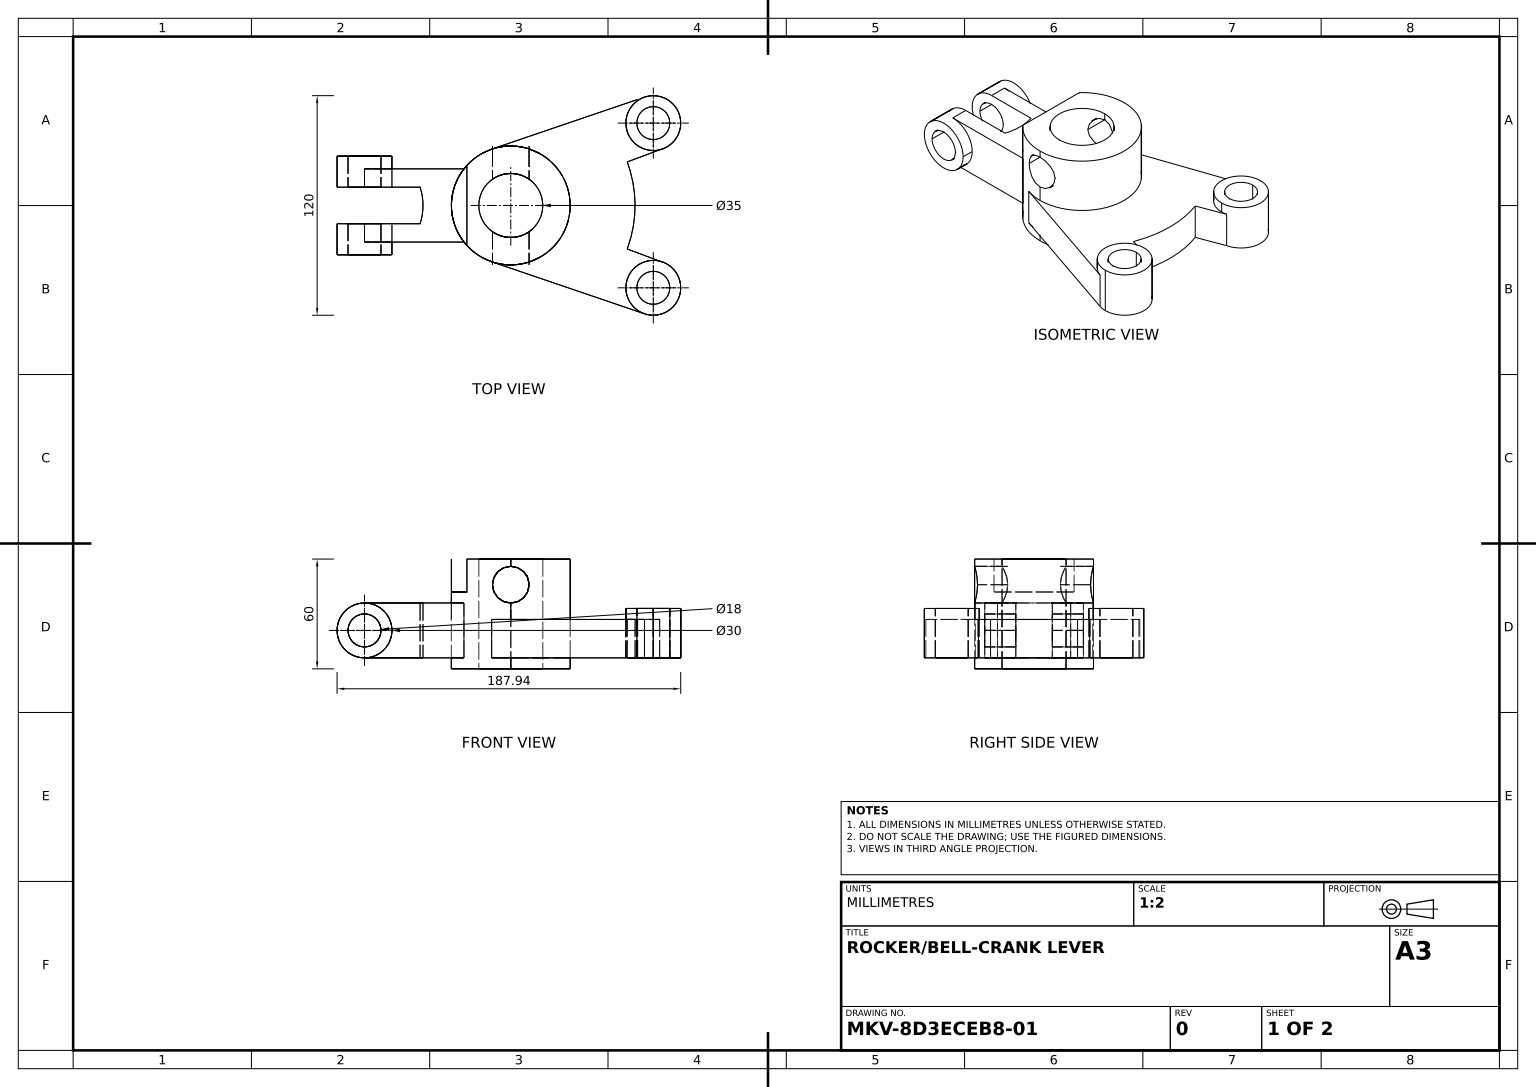
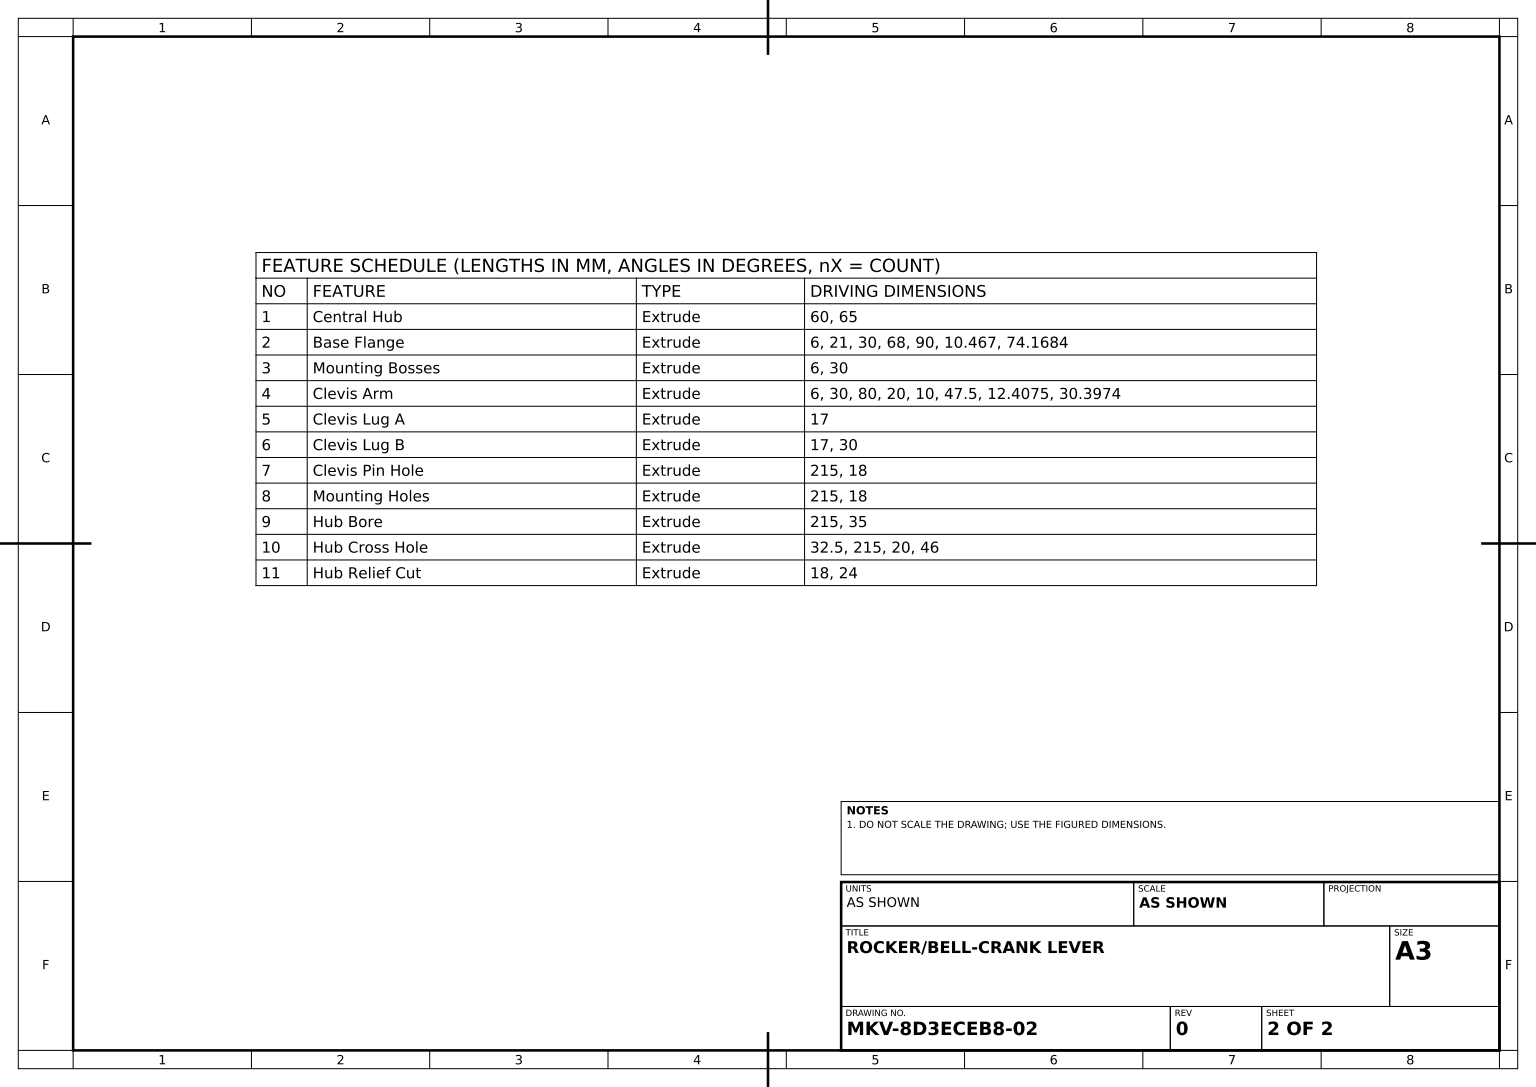
from build123d import *

# Parameters (mm, degrees)
HUB_PROFILE_SKETCH_R     = 32.5
CENTRAL_HUB_DEPTH        = 60
BASE_FLANGE_DEPTH        = 21
MOUNTING_BOSSES_SKETCH_R = 15
MOUNTING_BOSSES_DEPTH    = 6
CLEVIS_ARM_DEPTH         = 30
CLEVIS_LUG_A_SKETCH_R    = 15
CLEVIS_LUG_A_DEPTH       = 17
CLEVIS_START             = -17
CLEVIS_LUG_B_SKETCH_R    = 15
CLEVIS_LUG_B_DEPTH       = 17
CLEVIS_PIN_HOLE_SKETCH_R = 9
CLEVIS_PIN_HOLE_DEPTH    = 215
MOUNTING_HOLES_SKETCH_R  = 9
MOUNTING_HOLES_DEPTH     = 215
HUB_BORE_SKETCH_R        = 17.5
HUB_BORE_DEPTH           = 215
HUB_CROSS_HOLE_SKETCH_R  = 10
HUB_CROSS_HOLE_DEPTH     = 215
HUB_START                = -18
HUB_RELIEF_CUT_DEPTH     = 18


with BuildPart() as part:
    # Hub Profile Sketch → Central Hub (new body)
    with BuildSketch(Plane(origin=(0, 0, 0), x_dir=(1, 0, 0), z_dir=(0, 1, 0))):
        with Locations(Location((0, 0, 0), (0, 0, 270))):
            Circle(HUB_PROFILE_SKETCH_R)
    extrude(amount=CENTRAL_HUB_DEPTH)

    # Base Flange Sketch → Base Flange (add)
    with BuildSketch(Plane(origin=(0, 6, 0), x_dir=(1, 0, 0), z_dir=(0, 1, 0))):
        with BuildLine():
            Line((68.988226854, 57.798136264), (-10.467045475, 30.768343456))
            ThreePointArc((-10.467045475, 30.768343456), (32.5, 0), (-10.467045475, -30.768343456))
            Line((-10.467045475, -30.768343456), (73.111342275, -59.200773903))
            ThreePointArc((73.111342275, -59.200773903), (92.357418682, -49.147765612), (81.39742245, -30.40335537))
            Line((81.39742245, -30.40335537), (63.701379755, -23.793575127))
            ThreePointArc((63.701379755, -23.793575127), (68, 0), (63.701379755, 23.793575127))
            Line((63.701379755, 23.793575127), (81.39742245, 30.40335537))
            ThreePointArc((81.39742245, 30.40335537), (91.640276267, 51.112697602), (69.385841621, 57.320196986))
            ThreePointArc((69.385841621, 57.320196986), (69.187446933, 57.559509961), (68.988226854, 57.798136264))
        make_face()
    extrude(amount=BASE_FLANGE_DEPTH)

    # Mounting Bosses Sketch → Mounting Bosses (add)
    with BuildSketch(Plane(origin=(0, 27, 0), x_dir=(1, 0, 0), z_dir=(0, 1, 0))):
        with Locations(Location((77.942286341, 45, 0), (0, 0, 124.780191847))):
            Circle(MOUNTING_BOSSES_SKETCH_R)
        with Locations(Location((77.942286341, -45, 0), (0, 0, 76.682768473))):
            Circle(MOUNTING_BOSSES_SKETCH_R)
    extrude(amount=MOUNTING_BOSSES_DEPTH)

    # Clevis Arm Sketch → Clevis Arm (add)
    with BuildSketch(Plane(origin=(0, 6, 0), x_dir=(1, 0, 0), z_dir=(0, 1, 0))):
        with BuildLine():
            ThreePointArc((-49.602631693, -10), (-48, 0), (-49.602631693, 10))
            Line((-49.602631693, 10), (-80, 10))
            Line((-80, 10), (-80, 20))
            Line((-80, 20), (-32.5, 20))
            Line((-32.5, 20), (-20.092522132, 20))
            Line((-20.092522132, 20), (-20.092522132, -20))
            Line((-20.092522132, -20), (-32.5, -20))
            Line((-32.5, -20), (-80, -20))
            Line((-80, -20), (-80, -10))
            Line((-80, -10), (-49.602631693, -10))
        make_face()
    extrude(amount=CLEVIS_ARM_DEPTH)

    # Clevis Lug A Sketch → Clevis Lug A (add)
    with BuildSketch(Plane(origin=(0, 0, 10), x_dir=(-1, 0, 0), z_dir=(0, 0, -1))):
        with Locations((80, 21)):
            Circle(CLEVIS_LUG_A_SKETCH_R)
    extrude(amount=-CLEVIS_LUG_A_DEPTH)

    # Clevis Lug B Sketch → Clevis Lug B (add)
    with BuildSketch(Plane.XY.offset(-10).offset(CLEVIS_START)):
        with Locations(Location((-80, 21, 0), (0, 0, 180))):
            Circle(CLEVIS_LUG_B_SKETCH_R)
    extrude(amount=CLEVIS_LUG_B_DEPTH)

    # Clevis Pin Hole Sketch → Clevis Pin Hole (cut)
    with BuildSketch(Plane.XY.offset(27)):
        with Locations((-80, 21)):
            Circle(CLEVIS_PIN_HOLE_SKETCH_R)
    extrude(amount=-CLEVIS_PIN_HOLE_DEPTH, mode=Mode.SUBTRACT)

    # Mounting Holes Sketch → Mounting Holes (cut)
    with BuildSketch(Plane(origin=(0, 33, 0), x_dir=(1, 0, 0), z_dir=(0, 1, 0))):
        with Locations(Location((77.942286341, 45, 0), (0, 0, 270))):
            Circle(MOUNTING_HOLES_SKETCH_R)
        with Locations(Location((77.942286341, -45, 0), (0, 0, 270))):
            Circle(MOUNTING_HOLES_SKETCH_R)
    extrude(amount=-MOUNTING_HOLES_DEPTH, mode=Mode.SUBTRACT)

    # Hub Bore Sketch → Hub Bore (cut)
    with BuildSketch(Plane(origin=(0, 60, 0), x_dir=(1, 0, 0), z_dir=(0, 1, 0))):
        with Locations(Location((0, 0, 0), (0, 0, 270))):
            Circle(HUB_BORE_SKETCH_R)
    extrude(amount=-HUB_BORE_DEPTH, mode=Mode.SUBTRACT)

    # Hub Cross Hole Sketch → Hub Cross Hole (cut)
    with BuildSketch(Plane.XY.offset(32.5)):
        with Locations((0, 46)):
            Circle(HUB_CROSS_HOLE_SKETCH_R)
    extrude(amount=-HUB_CROSS_HOLE_DEPTH, mode=Mode.SUBTRACT)

    # Hub Relief Cut Sketch → Hub Relief Cut (cut)
    with BuildSketch(Plane(origin=(0, 60, 0), x_dir=(1, 0, 0), z_dir=(0, 1, 0)).offset(HUB_START)):
        with BuildLine():
            Line((-24, 0), (-24, 21.914607001))
            ThreePointArc((-24, 21.914607001), (-32.5, 0), (-24, -21.914607001))
            Line((-24, -21.914607001), (-24, 0))
        make_face()
    extrude(amount=HUB_RELIEF_CUT_DEPTH, mode=Mode.SUBTRACT)


solid = part.part
